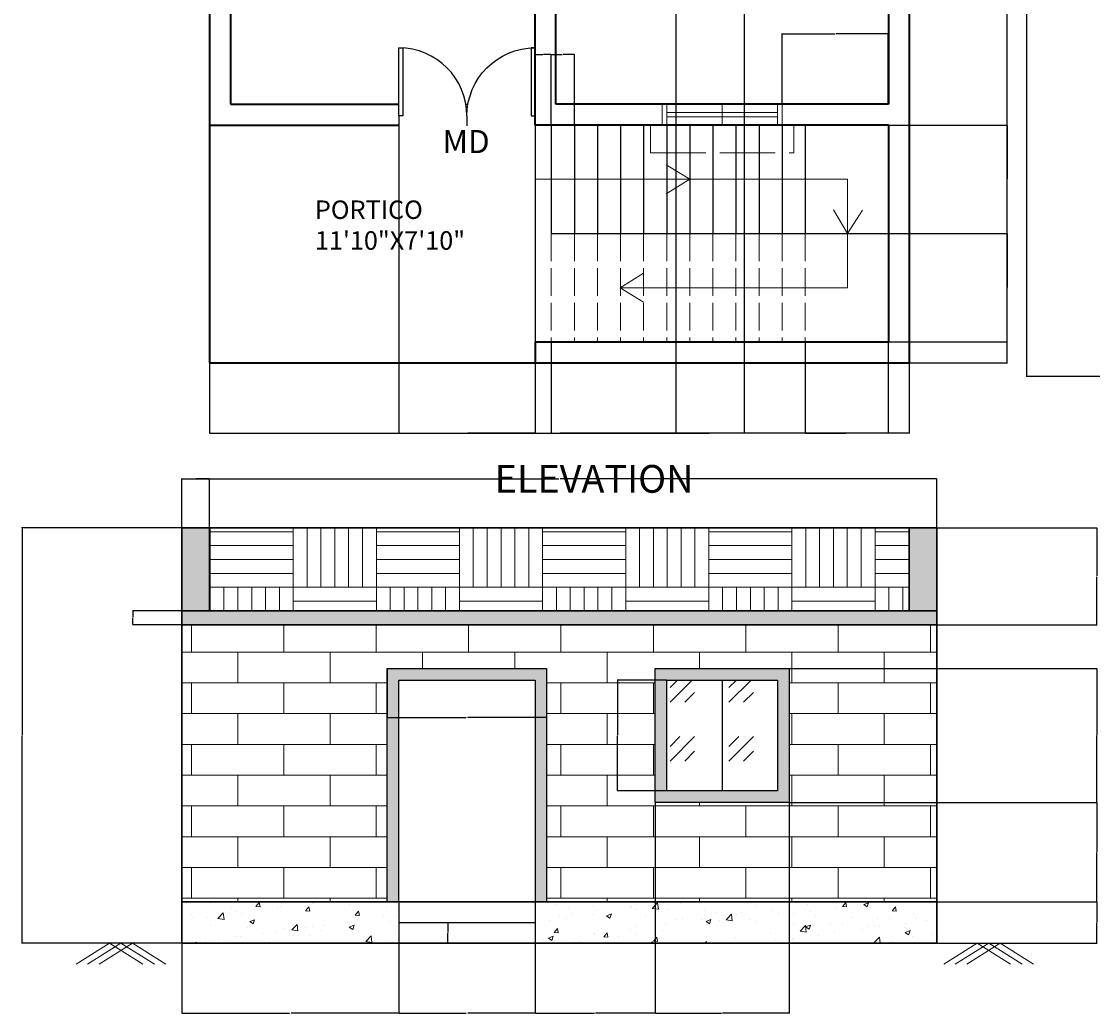
# Model space of a CAD drawing. Units: inches. Extents: x -154 to 668, y -797 to 97.
# Tile 1 of 4: x -154 to 313, y -797 to -367. Entities that reach past the tile are written whole.
import ezdxf

# ---------------------------------------------------------------- set-up
doc = ezdxf.new("R2010")
doc.units = ezdxf.units.IN
doc.header["$MEASUREMENT"] = 0
doc.linetypes.add('ACAD_ISO02W100', pattern=[15, 12, -3])
for name, color, linetype, lineweight in [('A-ANNO-DIMS', 2, 'Continuous', 18), ('A-ANNO-IDEN', 7, 'Continuous', 18), ('A-ANNO-SYMB', 7, 'Continuous', 18), ('A-ANNO-TITL', 1, 'Continuous', 30), ('A-AREA-IDEN', 7, 'Continuous', 18), ('A-DOOR', 7, 'Continuous', 25), ('A-ELEV', 3, 'Continuous', 30), ('A-ELEV-GRAD', 3, 'Continuous', 18), ('A-ELEV-OPEN', 3, 'Continuous', 25), ('A-ELEV-PATT', 2, 'Continuous', 13), ('A-FLOR-STRS', 220, 'Continuous', 25), ('A-FLOR-STRS-HIDN', 220, 'ACAD_ISO02W100', 18), ('A-GLAZ', 220, 'Continuous', 18), ('A-GLAZ-OVHD', 220, 'ACAD_ISO02W100', 13), ('A-WALL', 4, 'Continuous', 35)]:
    doc.layers.add(name, color=color, linetype=linetype, lineweight=lineweight)
doc.styles.get("Standard").update_dxf_attribs({"font": 'arial.ttf'})
doc.dimstyles.get("Standard").update_dxf_attribs({"dimtxt": 0.18, "dimasz": 0.18, "dimexe": 0.18, "dimexo": 0.0625, "dimgap": 0.09, "dimtad": 0, "dimtih": 1, "dimtoh": 1, "dimdec": 1, "dimzin": 0, "dimdsep": 46, "dimlunit": 4, "dimtxsty": 'Standard', "dimcen": 0.09, "dimadec": 0, "dimazin": 0, "dimtfac": 1, "dimtdec": 1, "dimtofl": 0, "dimtmove": 0, "dimatfit": 3, "dimfxl": 1, "dimtolj": 1, "dimtzin": 0, "dimarcsym": 0})

# ---------------------------------------------------------------- blocks, each defined once
blk = doc.blocks.new('*U5')
for p, q in [((0, 0), (0, -100)), ((750, 0), (750, -100))]:
    blk.add_line(p, q)
blk.add_lwpolyline([(0, 0), (0, 750), (43.75, 750), (43.75, 0)], close=True)
blk.add_arc((0, 0), 750, 0, 90)
blk = doc.blocks.new('WINDOW-48IN')
for p, q in [((-26, -4.5), (-26, 4.5)), ((-24, -4.5), (-24, 4.5)), ((-24, 1), (24, 1)), ((0, -4.5), (0, 4.5)), ((24, -4.5), (24, 4.5)), ((26, -4.5), (26, 4.5)), ((-24, -1), (24, -1))]:
    blk.add_line(p, q)
blk = doc.blocks.new('WINDOW-SHADE-48IN')
at = {"ltscale": 2}
for p, q in [((-31, -6), (-31, 6)), ((31, 6), (-31, 6)), ((31, -6), (31, 6)), ((-26, -6), (-31, -6)), ((26, -6), (31, -6))]:
    blk.add_line(p, q, dxfattribs=at)
blk = doc.blocks.new('GRADE-MARK')
for p, q in [((-5, 4.49), (-19.46, -4.49)), ((0, 4.49), (-14.46, -4.49)), ((5, 4.49), (-9.46, -4.49)), ((-5, 4.49), (9.46, -4.49)), ((0, 4.49), (14.46, -4.49)), ((5, 4.49), (19.46, -4.49))]:
    blk.add_line(p, q)
blk = doc.blocks.new('*D27')
at = {"layer": 'A-ANNO-DIMS', "color": 0, "lineweight": -2, "transparency": 16777216}
for p, q in [((-72.2, -514.8), (-72.2, -545.42)), ((230.8, -514.8), (230.8, -545.42)), ((-72.02, -545.24), (79.02, -545.24)), ((230.62, -545.24), (79.59, -545.24))]:
    blk.add_line(p, q, dxfattribs=at)
at = {"layer": 'A-ANNO-DIMS', "color": 0, "transparency": 16777216}
for points in [[(-72.02, -545.21), (-72.02, -545.27), (-72.2, -545.24)], [(230.62, -545.21), (230.62, -545.27), (230.8, -545.24)]]:
    blk.add_solid(points, dxfattribs=at)
at = {"layer": 'Defpoints', "color": 0, "transparency": 16777216}
for p in [(-72.2, -514.74), (230.8, -514.74), (230.8, -545.24)]:
    blk.add_point(p, dxfattribs=at)
at = {"layer": 'A-ANNO-DIMS', "color": 0, "transparency": 16777216, "insert": (79.3, -545.24), "char_height": 0.18, "attachment_point": 5}
blk.add_mtext('\\A1;303', dxfattribs=at)
blk = doc.blocks.new('*D28')
at = {"layer": 'A-ANNO-DIMS', "color": 0, "lineweight": -2, "transparency": 16777216}
for p, q in [((230.87, 51.26), (273.48, 51.26)), ((273.3, 51.08), (273.3, -231.56)), ((273.3, -514.56), (273.3, -231.92)), ((230.87, -514.74), (273.48, -514.74))]:
    blk.add_line(p, q, dxfattribs=at)
at = {"layer": 'A-ANNO-DIMS', "color": 0, "transparency": 16777216}
for points in [[(273.27, 51.08), (273.33, 51.08), (273.3, 51.26)], [(273.27, -514.56), (273.33, -514.56), (273.3, -514.74)]]:
    blk.add_solid(points, dxfattribs=at)
at = {"layer": 'Defpoints', "color": 0, "transparency": 16777216}
for p in [(230.8, 51.26), (273.3, 51.26), (230.8, -514.74)]:
    blk.add_point(p, dxfattribs=at)
at = {"layer": 'A-ANNO-DIMS', "color": 0, "transparency": 16777216, "insert": (273.3, -231.74), "char_height": 0.18, "attachment_point": 5}
blk.add_mtext('\\A1;566', dxfattribs=at)
blk = doc.blocks.new('*D29')
at = {"layer": 'A-ANNO-DIMS', "color": 0, "lineweight": -2, "transparency": 16777216}
for p, q in [((9.75, -411.8), (9.75, -545.42)), ((68.8, -411.8), (68.8, -545.42)), ((9.93, -545.24), (38.88, -545.24)), ((68.62, -545.24), (39.67, -545.24))]:
    blk.add_line(p, q, dxfattribs=at)
at = {"layer": 'A-ANNO-DIMS', "color": 0, "transparency": 16777216}
for points in [[(9.93, -545.21), (9.93, -545.27), (9.75, -545.24)], [(68.62, -545.21), (68.62, -545.27), (68.8, -545.24)]]:
    blk.add_solid(points, dxfattribs=at)
at = {"layer": 'Defpoints', "color": 0, "transparency": 16777216}
for p in [(9.75, -411.74), (68.8, -411.74), (68.8, -545.24)]:
    blk.add_point(p, dxfattribs=at)
at = {"layer": 'A-ANNO-DIMS', "color": 0, "transparency": 16777216, "insert": (39.28, -545.24), "char_height": 0.18, "attachment_point": 5}
blk.add_mtext('\\A1;59.06', dxfattribs=at)
blk = doc.blocks.new('*D38')
at = {"layer": 'A-ANNO-DIMS', "color": 0, "lineweight": -2, "transparency": 16777216}
for p, q in [((129.8, -258.8), (129.8, -545.42)), ((159.33, -258.8), (159.33, -545.42)), ((129.98, -545.24), (144.17, -545.24)), ((159.15, -545.24), (144.96, -545.24))]:
    blk.add_line(p, q, dxfattribs=at)
at = {"layer": 'A-ANNO-DIMS', "color": 0, "transparency": 16777216}
for points in [[(129.98, -545.21), (129.98, -545.27), (129.8, -545.24)], [(159.15, -545.21), (159.15, -545.27), (159.33, -545.24)]]:
    blk.add_solid(points, dxfattribs=at)
at = {"layer": 'Defpoints', "color": 0, "transparency": 16777216}
for p in [(129.8, -258.74), (159.33, -258.74), (159.33, -545.24)]:
    blk.add_point(p, dxfattribs=at)
at = {"layer": 'A-ANNO-DIMS', "color": 0, "transparency": 16777216, "insert": (144.57, -545.24), "char_height": 0.18, "attachment_point": 5}
blk.add_mtext('\\A1;29.53', dxfattribs=at)
blk = doc.blocks.new('*D43')
at = {"layer": 'A-ANNO-DIMS', "color": 0, "lineweight": -2, "transparency": 16777216}
for p, q in [((221.866879, -411.741585), (273.484379, -411.741585)), ((273.304379, -411.921585), (273.304379, -435.061585)), ((273.304379, -458.561585), (273.304379, -435.421585)), ((221.866879, -458.741585), (273.484379, -458.741585))]:
    blk.add_line(p, q, dxfattribs=at)
at = {"layer": 'A-ANNO-DIMS', "color": 0, "transparency": 16777216}
for points in [[(273.274379, -411.921585), (273.334379, -411.921585), (273.304379, -411.741585)], [(273.274379, -458.561585), (273.334379, -458.561585), (273.304379, -458.741585)]]:
    blk.add_solid(points, dxfattribs=at)
at = {"layer": 'Defpoints', "color": 0, "transparency": 16777216}
for p in [(221.804379, -411.741585), (273.304379, -411.741585), (221.804379, -458.741585)]:
    blk.add_point(p, dxfattribs=at)
at = {"layer": 'A-ANNO-DIMS', "color": 0, "transparency": 16777216, "insert": (273.304379, -435.241585), "char_height": 0.18, "attachment_point": 5}
blk.add_mtext('\\A1;47', dxfattribs=at)
blk = doc.blocks.new('*D44')
at = {"layer": 'A-ANNO-DIMS', "color": 0, "lineweight": -2, "transparency": 16777216}
for p, q in [((221.866879, -458.741585), (273.484379, -458.741585)), ((273.304379, -458.921585), (273.304379, -482.061585)), ((273.304379, -505.561585), (273.304379, -482.421585)), ((221.866879, -505.741585), (273.484379, -505.741585))]:
    blk.add_line(p, q, dxfattribs=at)
at = {"layer": 'A-ANNO-DIMS', "color": 0, "transparency": 16777216}
for points in [[(273.274379, -458.921585), (273.334379, -458.921585), (273.304379, -458.741585)], [(273.274379, -505.561585), (273.334379, -505.561585), (273.304379, -505.741585)]]:
    blk.add_solid(points, dxfattribs=at)
at = {"layer": 'Defpoints', "color": 0, "transparency": 16777216}
for p in [(221.804379, -458.741585), (273.304379, -458.741585), (221.804379, -505.741585)]:
    blk.add_point(p, dxfattribs=at)
at = {"layer": 'A-ANNO-DIMS', "color": 0, "transparency": 16777216, "insert": (273.304379, -482.241585), "char_height": 0.18, "attachment_point": 5}
blk.add_mtext('\\A1;47', dxfattribs=at)
blk = doc.blocks.new('*D45')
at = {"layer": 'A-ANNO-DIMS', "color": 0, "lineweight": -2, "transparency": 16777216}
for p, q in [((75.8, -411.68), (75.8, -381.06)), ((75.98, -381.24), (80.59, -381.24)), ((85.62, -381.24), (81.01, -381.24)), ((85.8, -411.68), (85.8, -381.06))]:
    blk.add_line(p, q, dxfattribs=at)
at = {"layer": 'A-ANNO-DIMS', "color": 0, "transparency": 16777216}
for points in [[(75.98, -381.21), (75.98, -381.27), (75.8, -381.24)], [(85.62, -381.21), (85.62, -381.27), (85.8, -381.24)]]:
    blk.add_solid(points, dxfattribs=at)
at = {"layer": 'Defpoints', "color": 0, "transparency": 16777216}
for p in [(85.8, -381.24), (75.8, -411.74), (85.8, -411.74)]:
    blk.add_point(p, dxfattribs=at)
at = {"layer": 'A-ANNO-DIMS', "color": 0, "transparency": 16777216, "insert": (80.8, -381.24), "char_height": 0.18, "attachment_point": 5}
blk.add_mtext('\\A1;10', dxfattribs=at)
blk = doc.blocks.new('*D46')
at = {"layer": 'A-ANNO-DIMS', "color": 0, "lineweight": -2, "transparency": 16777216}
for p, q in [((75.8, -505.8), (75.8, -545.42)), ((185.8, -505.8), (185.8, -545.42)), ((75.98, -545.24), (130.52, -545.24)), ((185.62, -545.24), (131.08, -545.24))]:
    blk.add_line(p, q, dxfattribs=at)
at = {"layer": 'A-ANNO-DIMS', "color": 0, "transparency": 16777216}
for points in [[(75.98, -545.21), (75.98, -545.27), (75.8, -545.24)], [(185.62, -545.21), (185.62, -545.27), (185.8, -545.24)]]:
    blk.add_solid(points, dxfattribs=at)
at = {"layer": 'Defpoints', "color": 0, "transparency": 16777216}
for p in [(75.8, -505.74), (185.8, -505.74), (185.8, -545.24)]:
    blk.add_point(p, dxfattribs=at)
at = {"layer": 'A-ANNO-DIMS', "color": 0, "transparency": 16777216, "insert": (130.8, -545.24), "char_height": 0.18, "attachment_point": 5}
blk.add_mtext('\\A1;110', dxfattribs=at)
blk = doc.blocks.new('*D47')
at = {"layer": 'A-ANNO-DIMS', "color": 0, "lineweight": -2, "transparency": 16777216}
for p, q in [((185.8, -505.8), (185.8, -545.42)), ((221.8, -505.8), (221.8, -545.42)), ((185.98, -545.24), (203.59, -545.24)), ((221.62, -545.24), (204.02, -545.24))]:
    blk.add_line(p, q, dxfattribs=at)
at = {"layer": 'A-ANNO-DIMS', "color": 0, "transparency": 16777216}
for points in [[(185.98, -545.21), (185.98, -545.27), (185.8, -545.24)], [(221.62, -545.21), (221.62, -545.27), (221.8, -545.24)]]:
    blk.add_solid(points, dxfattribs=at)
at = {"layer": 'Defpoints', "color": 0, "transparency": 16777216}
for p in [(185.8, -505.74), (221.8, -505.74), (221.8, -545.24)]:
    blk.add_point(p, dxfattribs=at)
at = {"layer": 'A-ANNO-DIMS', "color": 0, "transparency": 16777216, "insert": (203.8, -545.24), "char_height": 0.18, "attachment_point": 5}
blk.add_mtext('\\A1;36', dxfattribs=at)
blk = doc.blocks.new('*D48')
at = {"layer": 'A-ANNO-DIMS', "color": 0, "lineweight": -2, "transparency": 16777216}
for p, q in [((68.8, -411.68), (68.8, -381.06)), ((68.98, -381.24), (72.16, -381.24)), ((75.62, -381.24), (72.45, -381.24)), ((75.8, -411.68), (75.8, -381.06))]:
    blk.add_line(p, q, dxfattribs=at)
at = {"layer": 'A-ANNO-DIMS', "color": 0, "transparency": 16777216}
for points in [[(68.98, -381.21), (68.98, -381.27), (68.8, -381.24)], [(75.62, -381.21), (75.62, -381.27), (75.8, -381.24)]]:
    blk.add_solid(points, dxfattribs=at)
at = {"layer": 'Defpoints', "color": 0, "transparency": 16777216}
for p in [(75.8, -381.24), (68.8, -411.74), (75.8, -411.74)]:
    blk.add_point(p, dxfattribs=at)
at = {"layer": 'A-ANNO-DIMS', "color": 0, "transparency": 16777216, "insert": (72.3, -381.24), "char_height": 0.18, "attachment_point": 5}
blk.add_mtext('\\A1;7', dxfattribs=at)
blk = doc.blocks.new('*D49')
at = {"layer": 'A-ANNO-DIMS', "color": 0, "lineweight": -2, "transparency": 16777216}
for p, q in [((175.8, -402.68), (175.8, -372.06)), ((175.98, -372.24), (198.58, -372.24)), ((221.62, -372.24), (199.03, -372.24)), ((221.8, -402.68), (221.8, -372.06))]:
    blk.add_line(p, q, dxfattribs=at)
at = {"layer": 'A-ANNO-DIMS', "color": 0, "transparency": 16777216}
for points in [[(175.98, -372.21), (175.98, -372.27), (175.8, -372.24)], [(221.62, -372.21), (221.62, -372.27), (221.8, -372.24)]]:
    blk.add_solid(points, dxfattribs=at)
at = {"layer": 'Defpoints', "color": 0, "transparency": 16777216}
for p in [(221.8, -372.24), (175.8, -402.74), (221.8, -402.74)]:
    blk.add_point(p, dxfattribs=at)
at = {"layer": 'A-ANNO-DIMS', "color": 0, "transparency": 16777216, "insert": (198.8, -372.24), "char_height": 0.18, "attachment_point": 5}
blk.add_mtext('\\A1;46', dxfattribs=at)
blk = doc.blocks.new('*D51')
at = {"layer": 'A-ANNO-DIMS', "color": 0, "lineweight": -2, "transparency": 16777216}
for p, q in [((313.34, 65.33), (281.57, 65.33)), ((281.75, 65.15), (281.75, -227.49)), ((281.75, -520.49), (281.75, -227.85)), ((313.34, -520.67), (281.57, -520.67))]:
    blk.add_line(p, q, dxfattribs=at)
at = {"layer": 'A-ANNO-DIMS', "color": 0, "transparency": 16777216}
for points in [[(281.72, 65.15), (281.78, 65.15), (281.75, 65.33)], [(281.72, -520.49), (281.78, -520.49), (281.75, -520.67)]]:
    blk.add_solid(points, dxfattribs=at)
at = {"layer": 'Defpoints', "color": 0, "transparency": 16777216}
for p in [(281.75, 65.33), (313.4, 65.33), (313.4, -520.67)]:
    blk.add_point(p, dxfattribs=at)
at = {"layer": 'A-ANNO-DIMS', "color": 0, "transparency": 16777216, "insert": (281.75, -227.67), "char_height": 0.18, "attachment_point": 5}
blk.add_mtext('\\A1;586', dxfattribs=at)
blk = doc.blocks.new('*D62')
at = {"layer": 'A-ANNO-DIMS', "color": 0, "lineweight": -2, "transparency": 16777216}
for p, q in [((-84.2, -586.18), (-84.2, -564.81)), ((-84.02, -564.99), (79.02, -564.99)), ((242.62, -564.99), (79.59, -564.99)), ((242.8, -586.18), (242.8, -564.81))]:
    blk.add_line(p, q, dxfattribs=at)
at = {"layer": 'A-ANNO-DIMS', "color": 0, "transparency": 16777216}
for points in [[(-84.02, -564.96), (-84.02, -565.02), (-84.2, -564.99)], [(242.62, -564.96), (242.62, -565.02), (242.8, -564.99)]]:
    blk.add_solid(points, dxfattribs=at)
at = {"layer": 'Defpoints', "color": 0, "transparency": 16777216}
for p in [(242.8, -564.99), (-84.2, -586.24), (242.8, -586.24)]:
    blk.add_point(p, dxfattribs=at)
at = {"layer": 'A-ANNO-DIMS', "color": 0, "transparency": 16777216, "insert": (79.3, -564.99), "char_height": 0.18, "attachment_point": 5}
blk.add_mtext('\\A1;327', dxfattribs=at)
blk = doc.blocks.new('*D63')
at = {"layer": 'A-ANNO-DIMS', "color": 0, "lineweight": -2, "transparency": 16777216}
for p, q in [((-84.26, -586.24), (-153.63, -586.24)), ((-153.45, -586.42), (-153.45, -676.06)), ((-153.45, -766.06), (-153.45, -676.42)), ((-84.26, -766.24), (-153.63, -766.24))]:
    blk.add_line(p, q, dxfattribs=at)
at = {"layer": 'A-ANNO-DIMS', "color": 0, "transparency": 16777216}
for points in [[(-153.48, -586.42), (-153.42, -586.42), (-153.45, -586.24)], [(-153.48, -766.06), (-153.42, -766.06), (-153.45, -766.24)]]:
    blk.add_solid(points, dxfattribs=at)
at = {"layer": 'Defpoints', "color": 0, "transparency": 16777216}
for p in [(-153.45, -586.24), (-84.2, -586.24), (-84.2, -766.24)]:
    blk.add_point(p, dxfattribs=at)
at = {"layer": 'A-ANNO-DIMS', "color": 0, "transparency": 16777216, "insert": (-153.45, -676.24), "char_height": 0.18, "attachment_point": 5}
blk.add_mtext('\\A1;180', dxfattribs=at)
blk = doc.blocks.new('*D64')
at = {"layer": 'A-ANNO-DIMS', "color": 0, "lineweight": -2, "transparency": 16777216}
for p, q in [((242.87, -748.24), (312.23, -748.24)), ((312.05, -748.42), (312.05, -757.06)), ((312.05, -766.06), (312.05, -757.42)), ((242.87, -766.24), (312.23, -766.24))]:
    blk.add_line(p, q, dxfattribs=at)
at = {"layer": 'A-ANNO-DIMS', "color": 0, "transparency": 16777216}
for points in [[(312.02, -748.42), (312.08, -748.42), (312.05, -748.24)], [(312.02, -766.06), (312.08, -766.06), (312.05, -766.24)]]:
    blk.add_solid(points, dxfattribs=at)
at = {"layer": 'Defpoints', "color": 0, "transparency": 16777216}
for p in [(242.8, -748.24), (312.05, -748.24), (242.8, -766.24)]:
    blk.add_point(p, dxfattribs=at)
at = {"layer": 'A-ANNO-DIMS', "color": 0, "transparency": 16777216, "insert": (312.05, -757.24), "char_height": 0.18, "attachment_point": 5}
blk.add_mtext('\\A1;18', dxfattribs=at)
blk = doc.blocks.new('*D65')
at = {"layer": 'A-ANNO-DIMS', "color": 0, "lineweight": -2, "transparency": 16777216}
for p, q in [((242.87, -586.24), (312.23, -586.24)), ((312.05, -586.42), (312.05, -607.06)), ((312.05, -628.06), (312.05, -607.42)), ((242.87, -628.24), (312.23, -628.24))]:
    blk.add_line(p, q, dxfattribs=at)
at = {"layer": 'A-ANNO-DIMS', "color": 0, "transparency": 16777216}
for points in [[(312.02, -586.42), (312.08, -586.42), (312.05, -586.24)], [(312.02, -628.06), (312.08, -628.06), (312.05, -628.24)]]:
    blk.add_solid(points, dxfattribs=at)
at = {"layer": 'Defpoints', "color": 0, "transparency": 16777216}
for p in [(242.8, -586.24), (312.05, -586.24), (242.8, -628.24)]:
    blk.add_point(p, dxfattribs=at)
at = {"layer": 'A-ANNO-DIMS', "color": 0, "transparency": 16777216, "insert": (312.05, -607.24), "char_height": 0.18, "attachment_point": 5}
blk.add_mtext('\\A1;42', dxfattribs=at)
blk = doc.blocks.new('*D66')
at = {"layer": 'A-ANNO-DIMS', "color": 0, "lineweight": -2, "transparency": 16777216}
for p, q in [((-84.2, -766.3), (-84.2, -796.65)), ((9.75, -766.3), (9.75, -796.65)), ((-84.02, -796.47), (-37.62, -796.47)), ((9.57, -796.47), (-36.83, -796.47))]:
    blk.add_line(p, q, dxfattribs=at)
at = {"layer": 'A-ANNO-DIMS', "color": 0, "transparency": 16777216}
for points in [[(-84.02, -796.44), (-84.02, -796.5), (-84.2, -796.47)], [(9.57, -796.44), (9.57, -796.5), (9.75, -796.47)]]:
    blk.add_solid(points, dxfattribs=at)
at = {"layer": 'Defpoints', "color": 0, "transparency": 16777216}
for p in [(-84.2, -766.24), (9.75, -766.24), (9.75, -796.47)]:
    blk.add_point(p, dxfattribs=at)
at = {"layer": 'A-ANNO-DIMS', "color": 0, "transparency": 16777216, "insert": (-37.22, -796.47), "char_height": 0.18, "attachment_point": 5}
blk.add_mtext('\\A1;93.94', dxfattribs=at)
blk = doc.blocks.new('*D67')
at = {"layer": 'A-ANNO-DIMS', "color": 0, "lineweight": -2, "transparency": 16777216}
for p, q in [((9.75, -766.3), (9.75, -796.65)), ((68.8, -766.3), (68.8, -796.65)), ((9.93, -796.47), (38.88, -796.47)), ((68.62, -796.47), (39.67, -796.47))]:
    blk.add_line(p, q, dxfattribs=at)
at = {"layer": 'A-ANNO-DIMS', "color": 0, "transparency": 16777216}
for points in [[(9.93, -796.44), (9.93, -796.5), (9.75, -796.47)], [(68.62, -796.44), (68.62, -796.5), (68.8, -796.47)]]:
    blk.add_solid(points, dxfattribs=at)
at = {"layer": 'Defpoints', "color": 0, "transparency": 16777216}
for p in [(9.75, -766.24), (68.8, -766.24), (68.8, -796.47)]:
    blk.add_point(p, dxfattribs=at)
at = {"layer": 'A-ANNO-DIMS', "color": 0, "transparency": 16777216, "insert": (39.28, -796.47), "char_height": 0.18, "attachment_point": 5}
blk.add_mtext('\\A1;59.06', dxfattribs=at)
blk = doc.blocks.new('*D68')
at = {"layer": 'A-ANNO-DIMS', "color": 0, "lineweight": -2, "transparency": 16777216}
for p, q in [((120.8, -705.3), (120.8, -796.65)), ((68.8, -766.3), (68.8, -796.65)), ((68.98, -796.47), (94.59, -796.47)), ((120.62, -796.47), (95.02, -796.47))]:
    blk.add_line(p, q, dxfattribs=at)
at = {"layer": 'A-ANNO-DIMS', "color": 0, "transparency": 16777216}
for points in [[(68.98, -796.44), (68.98, -796.5), (68.8, -796.47)], [(120.62, -796.44), (120.62, -796.5), (120.8, -796.47)]]:
    blk.add_solid(points, dxfattribs=at)
at = {"layer": 'Defpoints', "color": 0, "transparency": 16777216}
for p in [(120.8, -705.24), (68.8, -766.24), (120.8, -796.47)]:
    blk.add_point(p, dxfattribs=at)
at = {"layer": 'A-ANNO-DIMS', "color": 0, "transparency": 16777216, "insert": (94.8, -796.47), "char_height": 0.18, "attachment_point": 5}
blk.add_mtext('\\A1;52', dxfattribs=at)
blk = doc.blocks.new('*D69')
at = {"layer": 'A-ANNO-DIMS', "color": 0, "lineweight": -2, "transparency": 16777216}
for p, q in [((120.8, -705.3), (120.8, -796.65)), ((178.8, -705.3), (178.8, -796.65)), ((120.98, -796.47), (149.59, -796.47)), ((178.62, -796.47), (150.02, -796.47))]:
    blk.add_line(p, q, dxfattribs=at)
at = {"layer": 'A-ANNO-DIMS', "color": 0, "transparency": 16777216}
for points in [[(120.98, -796.44), (120.98, -796.5), (120.8, -796.47)], [(178.62, -796.44), (178.62, -796.5), (178.8, -796.47)]]:
    blk.add_solid(points, dxfattribs=at)
at = {"layer": 'Defpoints', "color": 0, "transparency": 16777216}
for p in [(120.8, -705.24), (178.8, -705.24), (178.8, -796.47)]:
    blk.add_point(p, dxfattribs=at)
at = {"layer": 'A-ANNO-DIMS', "color": 0, "transparency": 16777216, "insert": (149.8, -796.47), "char_height": 0.18, "attachment_point": 5}
blk.add_mtext('\\A1;58', dxfattribs=at)
blk = doc.blocks.new('*D70')
at = {"layer": 'A-ANNO-DIMS', "color": 0, "lineweight": -2, "transparency": 16777216}
for p, q in [((178.87, -705.24), (312.23, -705.24)), ((312.05, -705.42), (312.05, -726.56)), ((312.05, -748.06), (312.05, -726.92)), ((242.87, -748.24), (312.23, -748.24))]:
    blk.add_line(p, q, dxfattribs=at)
at = {"layer": 'A-ANNO-DIMS', "color": 0, "transparency": 16777216}
for points in [[(312.02, -705.42), (312.08, -705.42), (312.05, -705.24)], [(312.02, -748.06), (312.08, -748.06), (312.05, -748.24)]]:
    blk.add_solid(points, dxfattribs=at)
at = {"layer": 'Defpoints', "color": 0, "transparency": 16777216}
for p in [(178.8, -705.24), (312.05, -705.24), (242.8, -748.24)]:
    blk.add_point(p, dxfattribs=at)
at = {"layer": 'A-ANNO-DIMS', "color": 0, "transparency": 16777216, "insert": (312.05, -726.74), "char_height": 0.18, "attachment_point": 5}
blk.add_mtext('\\A1;43', dxfattribs=at)
blk = doc.blocks.new('*D71')
at = {"layer": 'A-ANNO-DIMS', "color": 0, "lineweight": -2, "transparency": 16777216}
for p, q in [((178.87, -647.24), (312.23, -647.24)), ((312.05, -647.42), (312.05, -676.06)), ((312.05, -705.06), (312.05, -676.42)), ((178.87, -705.24), (312.23, -705.24))]:
    blk.add_line(p, q, dxfattribs=at)
at = {"layer": 'A-ANNO-DIMS', "color": 0, "transparency": 16777216}
for points in [[(312.02, -647.42), (312.08, -647.42), (312.05, -647.24)], [(312.02, -705.06), (312.08, -705.06), (312.05, -705.24)]]:
    blk.add_solid(points, dxfattribs=at)
at = {"layer": 'Defpoints', "color": 0, "transparency": 16777216}
for p in [(178.8, -647.24), (312.05, -647.24), (178.8, -705.24)]:
    blk.add_point(p, dxfattribs=at)
at = {"layer": 'A-ANNO-DIMS', "color": 0, "transparency": 16777216, "insert": (312.05, -676.24), "char_height": 0.18, "attachment_point": 5}
blk.add_mtext('\\A1;58', dxfattribs=at)
blk = doc.blocks.new('*D72')
at = {"layer": 'A-ANNO-DIMS', "color": 0, "lineweight": -2, "transparency": 16777216}
for p, q in [((-84.2, -586.18), (-84.2, -564.81)), ((-84.02, -564.99), (-78.41, -564.99)), ((-72.38, -564.99), (-77.99, -564.99)), ((-72.2, -586.18), (-72.2, -564.81))]:
    blk.add_line(p, q, dxfattribs=at)
at = {"layer": 'A-ANNO-DIMS', "color": 0, "transparency": 16777216}
for points in [[(-84.02, -564.96), (-84.02, -565.02), (-84.2, -564.99)], [(-72.38, -564.96), (-72.38, -565.02), (-72.2, -564.99)]]:
    blk.add_solid(points, dxfattribs=at)
at = {"layer": 'Defpoints', "color": 0, "transparency": 16777216}
for p in [(-72.2, -564.99), (-84.2, -586.24), (-72.2, -586.24)]:
    blk.add_point(p, dxfattribs=at)
at = {"layer": 'A-ANNO-DIMS', "color": 0, "transparency": 16777216, "insert": (-78.2, -564.99), "char_height": 0.18, "attachment_point": 5}
blk.add_mtext('\\A1;12', dxfattribs=at)
blk = doc.blocks.new('*D73')
at = {"layer": 'A-ANNO-DIMS', "color": 0, "lineweight": -2, "transparency": 16777216}
for p, q in [((-84.26, -622.24), (-105.63, -622.24)), ((-105.45, -622.42), (-105.45, -625.06)), ((-84.26, -628.24), (-105.63, -628.24)), ((-105.45, -628.06), (-105.45, -625.42))]:
    blk.add_line(p, q, dxfattribs=at)
at = {"layer": 'A-ANNO-DIMS', "color": 0, "transparency": 16777216}
for points in [[(-105.48, -622.42), (-105.42, -622.42), (-105.45, -622.24)], [(-105.48, -628.06), (-105.42, -628.06), (-105.45, -628.24)]]:
    blk.add_solid(points, dxfattribs=at)
at = {"layer": 'Defpoints', "color": 0, "transparency": 16777216}
for p in [(-105.45, -622.24), (-84.2, -622.24), (-84.2, -628.24)]:
    blk.add_point(p, dxfattribs=at)
at = {"layer": 'A-ANNO-DIMS', "color": 0, "transparency": 16777216, "insert": (-105.45, -625.24), "char_height": 0.18, "attachment_point": 5}
blk.add_mtext('\\A1;6', dxfattribs=at)
blk = doc.blocks.new('*D74')
at = {"layer": 'A-ANNO-DIMS', "color": 0, "lineweight": -2, "transparency": 16777216}
for p, q in [((125.74, -652.24), (104.37, -652.24)), ((104.55, -652.42), (104.55, -676.06)), ((104.55, -700.06), (104.55, -676.42)), ((125.74, -700.24), (104.37, -700.24))]:
    blk.add_line(p, q, dxfattribs=at)
at = {"layer": 'A-ANNO-DIMS', "color": 0, "transparency": 16777216}
for points in [[(104.52, -652.42), (104.58, -652.42), (104.55, -652.24)], [(104.52, -700.06), (104.58, -700.06), (104.55, -700.24)]]:
    blk.add_solid(points, dxfattribs=at)
at = {"layer": 'Defpoints', "color": 0, "transparency": 16777216}
for p in [(104.55, -652.24), (125.8, -652.24), (125.8, -700.24)]:
    blk.add_point(p, dxfattribs=at)
at = {"layer": 'A-ANNO-DIMS', "color": 0, "transparency": 16777216, "insert": (104.55, -676.24), "char_height": 0.18, "attachment_point": 5}
blk.add_mtext('\\A1;48', dxfattribs=at)
blk = doc.blocks.new('*D75')
at = {"layer": 'A-ANNO-DIMS', "color": 0, "lineweight": -2, "transparency": 16777216}
for p, q in [((9.81, -757.24), (31.18, -757.24)), ((31, -757.42), (31, -761.56)), ((31, -766.06), (31, -761.92)), ((9.81, -766.24), (31.18, -766.24))]:
    blk.add_line(p, q, dxfattribs=at)
at = {"layer": 'A-ANNO-DIMS', "color": 0, "transparency": 16777216}
for points in [[(30.97, -757.42), (31.03, -757.42), (31, -757.24)], [(30.97, -766.06), (31.03, -766.06), (31, -766.24)]]:
    blk.add_solid(points, dxfattribs=at)
at = {"layer": 'Defpoints', "color": 0, "transparency": 16777216}
for p in [(9.75, -757.24), (9.75, -766.24), (31, -766.24)]:
    blk.add_point(p, dxfattribs=at)
at = {"layer": 'A-ANNO-DIMS', "color": 0, "transparency": 16777216, "insert": (31, -761.74), "char_height": 0.18, "attachment_point": 5}
blk.add_mtext('\\A1;9', dxfattribs=at)
blk = doc.blocks.new('*D76')
at = {"layer": 'A-ANNO-DIMS', "color": 0, "lineweight": -2, "transparency": 16777216}
for p, q in [((4.75, -647.3), (4.75, -668.67)), ((73.8, -647.3), (73.8, -668.67)), ((4.93, -668.49), (38.88, -668.49)), ((73.62, -668.49), (39.67, -668.49))]:
    blk.add_line(p, q, dxfattribs=at)
at = {"layer": 'A-ANNO-DIMS', "color": 0, "transparency": 16777216}
for points in [[(4.93, -668.46), (4.93, -668.52), (4.75, -668.49)], [(73.62, -668.46), (73.62, -668.52), (73.8, -668.49)]]:
    blk.add_solid(points, dxfattribs=at)
at = {"layer": 'Defpoints', "color": 0, "transparency": 16777216}
for p in [(4.75, -647.24), (73.8, -647.24), (4.75, -668.49)]:
    blk.add_point(p, dxfattribs=at)
at = {"layer": 'A-ANNO-DIMS', "color": 0, "transparency": 16777216, "insert": (39.28, -668.49), "char_height": 0.18, "attachment_point": 5}
blk.add_mtext('\\A1;69.06', dxfattribs=at)

msp = doc.modelspace()

# ---------------------------------------------------------------- hatches: boundary and pattern name
at = {"layer": 'A-ELEV-PATT'}
h = msp.add_hatch(color=256, dxfattribs=at)
h.dxf.hatch_style = 1
h.paths.add_polyline_path([(-84.1956, -586.2406), (-84.1956, -622.2406), (242.8044, -622.2406), (242.8044, -586.2406)])
h.paths.add_polyline_path([(230.8044, -586.2406), (-72.1956, -586.2406), (-72.1956, -622.2406), (230.8044, -622.2406)], flags=16)
h.paths.add_polyline_path([(242.8044, -622.2406), (-84.1956, -622.2406), (-84.1956, -628.2406), (242.8044, -628.2406)])
h = msp.add_hatch(dxfattribs=at)
h.set_pattern_fill('AR-PARQ1', color=256, scale=3)
h.paths.add_polyline_path([(230.8044, -586.2406), (-72.1956, -586.2406), (-72.1956, -622.2406), (230.8044, -622.2406)])
h = msp.add_hatch(dxfattribs=at)
h.set_pattern_fill('AR-BRSTD', color=256, scale=5)
h.paths.add_polyline_path([(4.7493, -647.2406), (73.8044, -647.2406), (73.8044, -748.2406), (242.8044, -748.2406), (242.8044, -628.2406), (-84.1956, -628.2406), (-84.1956, -748.2406), (4.7493, -748.2406)])
h.paths.add_polyline_path([(120.8044, -647.2406), (178.8044, -647.2406), (178.8044, -705.2406), (120.8044, -705.2406)], flags=16)
h.paths.add_polyline_path([(125.8044, -652.2406), (173.8044, -652.2406), (173.8044, -700.2406), (125.8044, -700.2406)], flags=0)
h = msp.add_hatch(color=256, dxfattribs=at)
h.dxf.hatch_style = 1
h.paths.add_polyline_path([(9.7493, -652.2406), (68.8044, -652.2406), (68.8044, -748.2406), (73.8044, -748.2406), (73.8044, -647.2406), (4.7493, -647.2406), (4.7493, -748.2406), (9.7493, -748.2406)])
h.paths.add_polyline_path([(178.8044, -647.2406), (120.8044, -647.2406), (120.8044, -705.2406), (178.8044, -705.2406)])
h.paths.add_polyline_path([(125.8044, -652.2406), (173.8044, -652.2406), (173.8044, -700.2406), (125.8044, -700.2406)], flags=16)
h = msp.add_hatch(dxfattribs=at)
h.set_pattern_fill('GOST_GLASS', color=256, scale=3)
h.set_pattern_definition([(45, (0, 0), (25.45584, -3e-15), [15, -21]), (45, (6.364, 0), (25.45584, -3e-15), [6, -30]), (45, (0, 6.364), (25.45584, -3e-15), [6, -30])])
h.paths.add_polyline_path([(149.8044, -652.2406), (125.8044, -652.2406), (125.8044, -700.2406), (149.8044, -700.2406)])
h.paths.add_polyline_path([(173.8044, -652.2406), (149.8044, -652.2406), (149.8044, -700.2406), (173.8044, -700.2406)])
h = msp.add_hatch(dxfattribs=at)
h.set_pattern_fill('AR-CONC', color=256, scale=3)
h.paths.add_polyline_path([(9.7493, -748.2406), (-84.1956, -748.2406), (-84.1956, -766.2406), (9.7493, -766.2406)])
h.paths.add_polyline_path([(242.8044, -748.2406), (68.8044, -748.2406), (68.8044, -766.2406), (242.8044, -766.2406)])

# ---------------------------------------------------------------- linework, layer by layer
at = {"layer": 'A-ANNO-SYMB'}
for p, q in [((135.8044, -435.2416), (125.6312, -428.9575)), ((68.8044, -435.2416), (204.1543, -435.2416)), ((135.8044, -435.2416), (125.6312, -441.5257)), ((204.1543, -435.2416), (204.1543, -482.2337)), ((204.1543, -458.7377), (198.0021, -448.4841)), ((204.1543, -458.7377), (210.5692, -448.6464)), ((105.6312, -482.2337), (115.8044, -475.9496)), ((204.1543, -482.2337), (105.6312, -482.2337)), ((105.6312, -482.2337), (115.8044, -488.5178))]:
    msp.add_line(p, q, dxfattribs=at)
at = {"layer": 'A-DOOR'}
for p, q in [((38.8395, -402.7416), (39.7141, -402.7416)), ((39.0132, -411.7416), (39.5405, -411.7416))]:
    msp.add_line(p, q, dxfattribs=at)
at = {"layer": 'A-ELEV'}
for p, q in [((-84.1956, -586.2406), (242.8044, -586.2406)), ((-72.1956, -622.0284), (-72.1956, -586.2406)), ((230.8044, -586.2406), (230.8044, -622.2406)), ((-84.1956, -622.2406), (242.8044, -622.2406)), ((-84.1956, -628.2406), (242.8044, -628.2406)), ((-84.1956, -748.2406), (242.8044, -748.2406)), ((-84.1956, -766.2406), (242.8044, -766.2406))]:
    msp.add_line(p, q, dxfattribs=at)
for points in [[(-84.1956, -586.2406), (242.8044, -586.2406), (242.8044, -622.2406), (-84.1956, -622.2406)], [(-84.1956, -622.2406), (242.8044, -622.2406), (242.8044, -628.2406), (-84.1956, -628.2406)], [(-84.1956, -628.2406), (242.8044, -628.2406), (242.8044, -748.2406), (-84.1956, -748.2406)], [(-84.1956, -748.2406), (242.8044, -748.2406), (242.8044, -766.2406), (-84.1956, -766.2406)]]:
    msp.add_lwpolyline(points, close=True, dxfattribs=at)
at = {"layer": 'A-ELEV-GRAD'}
for p, q in [((-84.1956, -766.2406), (-132.1956, -766.2406)), ((242.8044, -766.2406), (290.8044, -766.2406))]:
    msp.add_line(p, q, dxfattribs=at)
at = {"layer": 'A-ELEV-OPEN'}
for p, q in [((149.8044, -652.2406), (149.8044, -700.2406)), ((9.7493, -748.2406), (68.8044, -748.2406)), ((9.7493, -748.2406), (9.7493, -766.2406)), ((68.8044, -748.2406), (68.8044, -766.2406)), ((9.7493, -757.2406), (68.8044, -757.2406))]:
    msp.add_line(p, q, dxfattribs=at)
msp.add_lwpolyline([(4.7493, -748.2406), (4.7493, -647.2406), (73.8044, -647.2406), (73.8044, -748.2406)], dxfattribs=at)
for points in [[(120.8044, -647.2406), (178.8044, -647.2406), (178.8044, -705.2406), (120.8044, -705.2406)], [(9.7493, -652.2406), (68.8044, -652.2406), (68.8044, -748.2406), (9.7493, -748.2406)], [(125.8044, -652.2406), (173.8044, -652.2406), (173.8044, -700.2406), (125.8044, -700.2406)]]:
    msp.add_lwpolyline(points, close=True, dxfattribs=at)
at = {"layer": 'A-FLOR-STRS'}
for p, q in [((75.8044, -411.7416), (75.8044, -458.7416)), ((85.8044, -411.7416), (85.8044, -458.7416)), ((95.8044, -411.7416), (95.8044, -458.7416)), ((105.8044, -411.7416), (105.8044, -458.7416)), ((115.8044, -411.7416), (115.8044, -458.7416)), ((125.8044, -411.7416), (125.8044, -458.7416)), ((135.8044, -411.7416), (135.8044, -458.7416)), ((145.8044, -411.7416), (145.8044, -458.7416)), ((155.8044, -411.7416), (155.8044, -458.7416)), ((165.8044, -411.7416), (165.8044, -458.7416)), ((175.8044, -411.7416), (175.8044, -458.7416)), ((185.8044, -411.7416), (185.8044, -458.7416)), ((75.8044, -458.7416), (221.8044, -458.7416))]:
    msp.add_line(p, q, dxfattribs=at)
at = {"layer": 'A-FLOR-STRS-HIDN'}
for p, q in [((75.8044, -458.7416), (75.8044, -505.7416)), ((85.8044, -458.7416), (85.8044, -505.7416)), ((95.8044, -458.7416), (95.8044, -505.7416)), ((105.8044, -458.7416), (105.8044, -505.7416)), ((115.8044, -458.7416), (115.8044, -505.7416)), ((125.8044, -458.7416), (125.8044, -505.7416)), ((135.8044, -458.7416), (135.8044, -505.7416)), ((145.8044, -458.7416), (145.8044, -505.7416)), ((155.8044, -458.7416), (155.8044, -505.7416)), ((165.8044, -458.7416), (165.8044, -505.7416)), ((175.8044, -458.7416), (175.8044, -505.7416)), ((185.8044, -458.7416), (185.8044, -505.7416))]:
    msp.add_line(p, q, dxfattribs=at)
at = {"layer": 'A-WALL'}
for p, q in [((68.8044, -411.7416), (68.8044, -249.7416)), ((77.8044, -402.7416), (77.8044, -249.7416)), ((-72.1956, -258.7416), (-72.1956, -411.7416)), ((-63.1956, -258.7416), (-63.1956, -402.7416)), ((221.8044, -258.7416), (221.8044, -402.7416)), ((230.8044, -258.7416), (230.8044, -514.7416)), ((-63.1956, -402.7416), (9.7493, -402.7416)), ((221.8044, -402.7416), (77.8044, -402.7416)), ((-72.1956, -411.7416), (9.7493, -411.7416)), ((-72.1956, -411.7416), (-72.1956, -514.7416)), ((221.8044, -411.7416), (68.8044, -411.7416)), ((221.8044, -411.7416), (221.8044, -505.7416)), ((68.8044, -505.7416), (68.8044, -514.7416)), ((68.8044, -505.7416), (221.8044, -505.7416)), ((-72.1956, -514.7416), (230.8044, -514.7416))]:
    msp.add_line(p, q, dxfattribs=at)

# ---------------------------------------------------------------- block references
at = {"layer": 'A-DOOR', "yscale": 0.0393700787401575, "zscale": 0.0393700787401575}
for p, xscale in [((9.7493, -407.8046), 0.0393700787401575), ((68.8044, -407.8046), -0.0393700787401575)]:
    msp.add_blockref('*U5', p, dxfattribs=dict(at, xscale=xscale))
at = {"layer": 'A-ELEV-GRAD'}
for p in [(-110.584, -770.732), (265.2708, -770.732)]:
    msp.add_blockref('GRADE-MARK', p, dxfattribs=at)
at = {"layer": 'A-GLAZ'}
msp.add_blockref('WINDOW-48IN', (149.804, -407.242), dxfattribs=at)
at = {"layer": 'A-GLAZ-OVHD', "rotation": 180}
msp.add_blockref('WINDOW-SHADE-48IN', (149.8048, -417.7412), dxfattribs=at)

# ---------------------------------------------------------------- texts
at = {"layer": 'A-ANNO-IDEN'}
msp.add_text('MD', height=10, dxfattribs=at).set_placement((28.6645, -423.8941))
at = {"layer": 'A-ANNO-TITL'}
msp.add_text('ELEVATION', height=12, dxfattribs=at).set_placement((51.278, -571.0393))
at = {"layer": 'A-AREA-IDEN', "insert": (-26.5739, -444.4284), "char_height": 8, "attachment_point": 1}
msp.add_mtext_dynamic_manual_height_columns('PORTICO\\P11\'10"X7\'10"', width=87.70688, gutter_width=1, heights=[0], dxfattribs=at)

# ---------------------------------------------------------------- dimensions: what is measured, and where the dimension line sits
at = {"layer": 'A-ANNO-DIMS'}
for base, p1, p2, angle, override, picture, middle in [((281.7497, 65.3328), (313.3997, -520.6672), (313.3997, 65.3328), 90, {"dimdec": 0, "dimlfac": 1, "dimrnd": 0, "dimzin": 0, "dimdsep": 46, "dimlunit": 2}, '*D51', (281.7497, -227.6672)), ((273.3044, 51.2584), (230.8044, -514.7416), (230.8044, 51.2584), 90, {"dimdec": 0, "dimlfac": 1, "dimrnd": 0, "dimzin": 0, "dimdsep": 46, "dimlunit": 2}, '*D28', (273.3044, -231.7416)), ((273.3044, -411.7416), (221.8044, -458.7416), (221.8044, -411.7416), 90, {"dimdec": 0, "dimlfac": 1, "dimrnd": 0, "dimzin": 0, "dimdsep": 46, "dimlunit": 2}, '*D43', (273.3044, -435.2416)), ((273.3044, -458.7416), (221.8044, -505.7416), (221.8044, -458.7416), 90, {"dimdec": 0, "dimlfac": 1, "dimrnd": 0, "dimzin": 0, "dimdsep": 46, "dimlunit": 2}, '*D44', (273.3044, -482.2416)), ((-153.4456, -586.2406), (-84.1956, -766.2406), (-84.1956, -586.2406), 90, {"dimdec": 0, "dimlfac": 1, "dimrnd": 0, "dimzin": 0, "dimdsep": 46, "dimlunit": 2}, '*D63', (-153.4456, -676.2406)), ((312.0544, -586.2406), (242.8044, -628.2406), (242.8044, -586.2406), 90, {"dimdec": 0, "dimlfac": 1, "dimrnd": 0, "dimzin": 0, "dimdsep": 46, "dimlunit": 2}, '*D65', (312.0544, -607.2406)), ((-105.4456, -622.2406), (-84.1956, -628.2406), (-84.1956, -622.2406), 90, {"dimdec": 0, "dimlfac": 1, "dimrnd": 0, "dimzin": 0, "dimdsep": 46, "dimlunit": 2}, '*D73', (-105.4456, -625.2406)), ((4.7493, -668.4906), (73.8044, -647.2406), (4.7493, -647.2406), 180, {"dimdec": 2, "dimlfac": 1, "dimrnd": 0, "dimzin": 0, "dimdsep": 46, "dimlunit": 2}, '*D76', (39.2768, -668.4906)), ((312.0544, -647.2406), (178.8044, -705.2406), (178.8044, -647.2406), 90, {"dimdec": 0, "dimlfac": 1, "dimrnd": 0, "dimzin": 0, "dimdsep": 46, "dimlunit": 2}, '*D71', (312.0544, -676.2406)), ((104.5544, -652.2406), (125.8044, -700.2406), (125.8044, -652.2406), 90, {"dimdec": 0, "dimlfac": 1, "dimrnd": 0, "dimzin": 0, "dimdsep": 46, "dimlunit": 2}, '*D74', (104.5544, -676.2406)), ((312.0544, -705.2406), (242.8044, -748.2406), (178.8044, -705.2406), 90, {"dimdec": 0, "dimlfac": 1, "dimrnd": 0, "dimzin": 0, "dimdsep": 46, "dimlunit": 2}, '*D70', (312.0544, -726.7406)), ((312.0544, -748.2406), (242.8044, -766.2406), (242.8044, -748.2406), 90, {"dimdec": 0, "dimlfac": 1, "dimrnd": 0, "dimzin": 0, "dimdsep": 46, "dimlunit": 2}, '*D64', (312.0544, -757.2406)), ((30.9993, -766.2406), (9.7493, -757.2406), (9.7493, -766.2406), 270, {"dimdec": 0, "dimlfac": 1, "dimrnd": 0, "dimzin": 0, "dimdsep": 46, "dimlunit": 2}, '*D75', (30.9993, -761.7406))]:
    dim = msp.add_linear_dim(base=base, p1=p1, p2=p2, angle=angle, dimstyle='Standard', override=override, dxfattribs=at)
    dim.commit()
    dim.dimension.update_dxf_attribs({"geometry": picture, "text_midpoint": middle})
for base, p1, p2, override, picture, middle in [((159.3319, -545.2416), (129.8044, -258.7416), (159.3319, -258.7416), {"dimdec": 2, "dimlfac": 1, "dimrnd": 0, "dimzin": 0, "dimdsep": 46, "dimlunit": 2}, '*D38', (144.5682, -545.2416)), ((221.8044, -372.2416), (175.8044, -402.7416), (221.8044, -402.7416), {"dimdec": 0, "dimlfac": 1, "dimrnd": 0, "dimzin": 0, "dimdsep": 46, "dimlunit": 2}, '*D49', (198.8044, -372.2416)), ((75.8044, -381.2416), (68.8044, -411.7416), (75.8044, -411.7416), {"dimdec": 0, "dimlfac": 1, "dimrnd": 0, "dimzin": 0, "dimdsep": 46, "dimlunit": 2}, '*D48', (72.3044, -381.2416)), ((85.8044, -381.2416), (75.8044, -411.7416), (85.8044, -411.7416), {"dimdec": 0, "dimlfac": 1, "dimrnd": 0, "dimzin": 0, "dimdsep": 46, "dimlunit": 2}, '*D45', (80.8044, -381.2416)), ((68.8044, -545.2416), (9.7493, -411.7416), (68.8044, -411.7416), {"dimdec": 2, "dimlfac": 1, "dimrnd": 0, "dimzin": 0, "dimdsep": 46, "dimlunit": 2}, '*D29', (39.2768, -545.2416)), ((185.8044, -545.2416), (75.8044, -505.7416), (185.8044, -505.7416), {"dimdec": 0, "dimlfac": 1, "dimrnd": 0, "dimzin": 0, "dimdsep": 46, "dimlunit": 2}, '*D46', (130.8044, -545.2416)), ((221.8044, -545.2416), (185.8044, -505.7416), (221.8044, -505.7416), {"dimdec": 0, "dimlfac": 1, "dimrnd": 0, "dimzin": 0, "dimdsep": 46, "dimlunit": 2}, '*D47', (203.8044, -545.2416)), ((230.8044, -545.2416), (-72.1956, -514.7416), (230.8044, -514.7416), {"dimdec": 0, "dimlfac": 1, "dimrnd": 0, "dimzin": 0, "dimdsep": 46, "dimlunit": 2}, '*D27', (79.3044, -545.2416)), ((242.8044, -564.9906), (-84.1956, -586.2406), (242.8044, -586.2406), {"dimdec": 0, "dimlfac": 1, "dimrnd": 0, "dimzin": 0, "dimdsep": 46, "dimlunit": 2}, '*D62', (79.3044, -564.9906)), ((-72.1956, -564.9906), (-84.1956, -586.2406), (-72.1956, -586.2406), {"dimdec": 0, "dimlfac": 1, "dimrnd": 0, "dimzin": 0, "dimdsep": 46, "dimlunit": 2}, '*D72', (-78.1956, -564.9906)), ((120.8044, -796.4727), (68.8044, -766.2406), (120.8044, -705.2406), {"dimdec": 0, "dimlfac": 1, "dimrnd": 0, "dimzin": 0, "dimdsep": 46, "dimlunit": 2}, '*D68', (94.8044, -796.4727)), ((178.8044, -796.4727), (120.8044, -705.2406), (178.8044, -705.2406), {"dimdec": 0, "dimlfac": 1, "dimrnd": 0, "dimzin": 0, "dimdsep": 46, "dimlunit": 2}, '*D69', (149.8044, -796.4727)), ((9.7493, -796.4727), (-84.1956, -766.2406), (9.7493, -766.2406), {"dimdec": 2, "dimlfac": 1, "dimrnd": 0, "dimzin": 0, "dimdsep": 46, "dimlunit": 2}, '*D66', (-37.2232, -796.4727)), ((68.8044, -796.4727), (9.7493, -766.2406), (68.8044, -766.2406), {"dimdec": 2, "dimlfac": 1, "dimrnd": 0, "dimzin": 0, "dimdsep": 46, "dimlunit": 2}, '*D67', (39.2768, -796.4727))]:
    dim = msp.add_linear_dim(base=base, p1=p1, p2=p2, dimstyle='Standard', override=override, dxfattribs=at)
    dim.commit()
    dim.dimension.update_dxf_attribs({"geometry": picture, "text_midpoint": middle})

doc.saveas('drawing.dxf')
